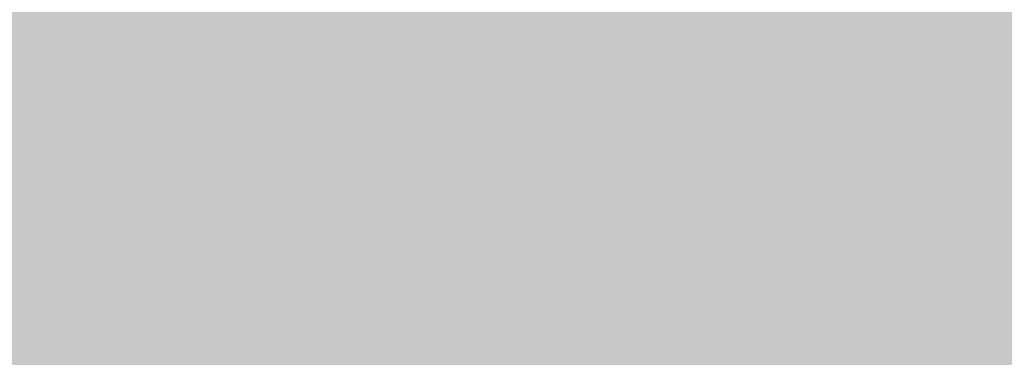
# Model space of a CAD drawing. Units: millimetres. Extents: x 0 to 2267, y 0 to 1823.
# Tile 74 of 256: x 1596.855 to 1600.369, y 1227.321 to 1228.528. Entities that reach past the tile are written whole.
import ezdxf

# ---------------------------------------------------------------- set-up
doc = ezdxf.new("R2010")
doc.units = ezdxf.units.MM
doc.header["$MEASUREMENT"] = 0
doc.layers.add('M-HATC', color=252, linetype='Continuous', lineweight=18)

msp = doc.modelspace()

# ---------------------------------------------------------------- hatches: boundary and pattern name
at = {"layer": 'M-HATC'}
h = msp.add_hatch(color=256, dxfattribs=at)
h.dxf.hatch_style = 1
h.paths.add_polyline_path([(2055.771, 1603.062), (1381.0868, 1603.062), (1381.0868, 1598.062), (2055.771, 1598.062)])
h.paths.add_polyline_path([(2055.771, 1598.062), (1381.0868, 1598.062), (1381.0868, 1593.062), (2055.771, 1593.062)])
h.paths.add_polyline_path([(2051.3074, 1536.7609), (1385.5504, 1536.7609), (1385.5504, 1526.7609), (1387.5504, 1526.7609), (1388.5366, 1525.0528), (1385.3319, 1521.2335), (1385.3319, 1521.2226), (2050.2542, 1522.7491), (2048.3212, 1525.0528), (2049.3074, 1526.7609), (2051.3074, 1526.7609)])
edge = h.paths.add_edge_path()
edge.add_arc((1847.5345, 1379.1492), 135, 222.603061, 222.890851, ccw=False)
edge.add_line((1748.1663, 1287.7656), (1683.0921, 1287.7656))
edge.add_arc((1583.7239, 1379.1492), 135, 317.109149, 317.396939, ccw=False)
edge.add_arc((1678.9686, 1290.6707), 5, 222.8909, 317.1091, ccw=False)
edge.add_arc((1774.2133, 1379.1492), 135, 222.603061, 222.890851, ccw=False)
edge.add_line((1674.8451, 1287.7656), (1609.7709, 1287.7656))
edge.add_arc((1510.4027, 1379.1492), 135, 317.109149, 317.396939, ccw=False)
edge.add_arc((1605.6474, 1290.6707), 5, 222.8909, 317.1091, ccw=False)
edge.add_arc((1700.8921, 1379.1492), 135, 222.603061, 222.890851, ccw=False)
edge.add_line((1601.5239, 1287.7656), (1536.4497, 1287.7656))
edge.add_arc((1437.0815, 1379.1492), 135, 317.109149, 317.396939, ccw=False)
edge.add_arc((1532.3262, 1290.6707), 5, 222.8909, 317.1091, ccw=False)
edge.add_arc((1627.5709, 1379.1492), 135, 222.603061, 222.890851, ccw=False)
edge.add_line((1528.2027, 1287.7656), (1505.9289, 1287.7656))
edge.add_spline(control_points=[(1505.9289, 1287.7656), (1504.2622, 1287.7656), (1504.2622, 1282.7656), (1505.9289, 1282.7656)], knot_values=[0, 0, 0, 0, 5, 5, 5, 5], degree=3, periodic=0)
edge.add_line((1505.9289, 1282.7656), (1930.9289, 1282.7656))
edge.add_spline(control_points=[(1930.9289, 1282.7656), (1932.5956, 1282.7656), (1932.5956, 1287.7656), (1930.9289, 1287.7656)], knot_values=[0, 0, 0, 0, 5, 5, 5, 5], degree=3, periodic=0)
edge.add_line((1930.9289, 1287.7656), (1903.0557, 1287.7656))
edge.add_arc((1803.6875, 1379.1492), 135, 317.109149, 317.396939, ccw=False)
edge.add_arc((1898.9322, 1290.6707), 5, 222.8909, 317.1091, ccw=False)
edge.add_arc((1994.1769, 1379.1492), 135, 222.603061, 222.890851, ccw=False)
edge.add_line((1894.8087, 1287.7656), (1829.7345, 1287.7656))
edge.add_arc((1730.3663, 1379.1492), 135, 317.109149, 317.396939, ccw=False)
edge.add_arc((1825.611, 1290.6707), 5, 222.8909, 317.1091, ccw=False)
edge.add_arc((1920.8557, 1379.1492), 135, 222.603061, 222.890851, ccw=False)
edge.add_line((1821.4875, 1287.7656), (1756.4133, 1287.7656))
edge.add_arc((1657.0451, 1379.1492), 135, 317.109149, 317.396939, ccw=False)
edge.add_arc((1752.2898, 1290.6707), 5, 222.8909, 317.1091, ccw=False)
edge = h.paths.add_edge_path()
edge.add_spline(control_points=[(1843.4289, 1227.2475), (1845.0956, 1227.2475), (1845.0956, 1232.2475), (1843.4289, 1232.2475)], knot_values=[0, 0, 0, 0, 5, 5, 5, 5], degree=3, periodic=0)
edge.add_line((1843.4289, 1232.2475), (1593.4289, 1232.2475))
edge.add_spline(control_points=[(1593.4289, 1232.2475), (1591.7622, 1232.2475), (1591.7622, 1227.2475), (1593.4289, 1227.2475)], knot_values=[0, 0, 0, 0, 5, 5, 5, 5], degree=3, periodic=0)
edge.add_line((1593.4289, 1227.2475), (1843.4289, 1227.2475))
h.paths.add_polyline_path([(1905.9289, 1127.4171), (1530.9289, 1127.4171, 0.414214), (1520.9289, 1117.4171), (1530.9289, 1117.4171), (1915.9289, 1117.4171, 0.414214)])
edge = h.paths.add_edge_path()
edge.add_arc((1397.0858, 1498.4078), 12.7299, 90.78215, 190.87871, ccw=False)
edge.add_line((1396.912, 1511.1365), (1428.0097, 1511.3488))
edge.add_line((1428.0097, 1511.3488), (1433.0097, 1511.3488))
edge.add_line((1433.0097, 1511.3488), (1434.439, 1511.3488))
edge.add_arc((1419.474, 1498.0804), 20, 41.561, 74.08211)
edge.add_line((1424.9592, 1517.3135), (1399.9351, 1517.2561))
edge.add_spline(control_points=[(1399.9307, 1517.2561), (1399.884, 1517.2131), (1399.8328, 1517.1689), (1399.7774, 1517.1236)], knot_values=[11.567499, 11.567499, 11.567499, 11.567499, 11.814249, 11.814249, 11.814249, 11.814249], degree=3, periodic=0)
edge.add_spline(control_points=[(1399.6328, 1517.0099), (1399.5831, 1516.9721), (1399.5307, 1516.9338), (1399.4759, 1516.8947)], knot_values=[11.167718, 11.167718, 11.167718, 11.167718, 11.365188, 11.365188, 11.365188, 11.365188], degree=3, periodic=0)
edge.add_spline(control_points=[(1399.3398, 1516.8001), (1399.1514, 1516.6719), (1398.9384, 1516.5377), (1398.704, 1516.3994)], knot_values=[10.376405, 10.376405, 10.376405, 10.376405, 11.00994, 11.00994, 11.00994, 11.00994], degree=3, periodic=0)
edge.add_spline(control_points=[(1398.6572, 1516.3719), (1398.5789, 1516.326), (1398.4983, 1516.2797), (1398.4155, 1516.2331)], knot_values=[10.125175, 10.125175, 10.125175, 10.125175, 10.334406, 10.334406, 10.334406, 10.334406], degree=3, periodic=0)
edge.add_spline(control_points=[(1398.2642, 1516.1487), (1398.196, 1516.1111), (1398.1263, 1516.0732), (1398.0555, 1516.0351)], knot_values=[9.832246, 9.832246, 9.832246, 9.832246, 9.999658, 9.999658, 9.999658, 9.999658], degree=3, periodic=0)
edge.add_spline(control_points=[(1397.9987, 1516.0048), (1397.7312, 1515.8621), (1397.446, 1515.7171), (1397.1466, 1515.5714)], knot_values=[9.161808, 9.161808, 9.161808, 9.161808, 9.787769, 9.787769, 9.787769, 9.787769], degree=3, periodic=0)
edge.add_spline(control_points=[(1397.1466, 1515.5714), (1396.8418, 1515.423), (1396.5222, 1515.274), (1396.1914, 1515.1262)], knot_values=[8.524455, 8.524455, 8.524455, 8.524455, 9.161808, 9.161808, 9.161808, 9.161808], degree=3, periodic=0)
edge.add_spline(control_points=[(1396.0777, 1515.0756), (1395.9854, 1515.0348), (1395.8922, 1514.994), (1395.7983, 1514.9534)], knot_values=[8.275193, 8.275193, 8.275193, 8.275193, 8.451726, 8.451726, 8.451726, 8.451726], degree=3, periodic=0)
edge.add_spline(control_points=[(1395.6018, 1514.8691), (1395.4997, 1514.8257), (1395.3968, 1514.7824), (1395.2932, 1514.7394)], knot_values=[7.962917, 7.962917, 7.962917, 7.962917, 8.152764, 8.152764, 8.152764, 8.152764], degree=3, periodic=0)
edge.add_spline(control_points=[(1395.2116, 1514.7057), (1394.8278, 1514.5475), (1394.4345, 1514.3929), (1394.0364, 1514.2442)], knot_values=[7.21254, 7.21254, 7.21254, 7.21254, 7.913148, 7.913148, 7.913148, 7.913148], degree=3, periodic=0)
edge.add_spline(control_points=[(1394.0364, 1514.2442), (1393.7076, 1514.1214), (1393.3754, 1514.0027), (1393.0427, 1513.8895)], knot_values=[6.633733, 6.633733, 6.633733, 6.633733, 7.21254, 7.21254, 7.21254, 7.21254], degree=3, periodic=0)
edge.add_spline(control_points=[(1392.8214, 1513.815), (1392.7198, 1513.7812), (1392.6181, 1513.7479), (1392.5166, 1513.7152)], knot_values=[6.328796, 6.328796, 6.328796, 6.328796, 6.505493, 6.505493, 6.505493, 6.505493], degree=3, periodic=0)
edge.add_spline(control_points=[(1392.5166, 1513.7152), (1392.3187, 1513.6515), (1392.1212, 1513.59), (1391.9244, 1513.531)], knot_values=[5.984605, 5.984605, 5.984605, 5.984605, 6.328796, 6.328796, 6.328796, 6.328796], degree=3, periodic=0)
edge.add_spline(control_points=[(1391.7915, 1513.4915), (1391.3122, 1513.3501), (1390.8384, 1513.2239), (1390.3784, 1513.1171)], knot_values=[5.066697, 5.066697, 5.066697, 5.066697, 5.907055, 5.907055, 5.907055, 5.907055], degree=3, periodic=0)
edge.add_spline(control_points=[(1390.3784, 1513.1171), (1390.1797, 1513.071), (1389.9836, 1513.0284), (1389.7907, 1512.9899)], knot_values=[4.70367, 4.70367, 4.70367, 4.70367, 5.066695, 5.066695, 5.066695, 5.066695], degree=3, periodic=0)
edge.add_spline(control_points=[(1389.422, 1512.9204), (1389.2459, 1512.8892), (1389.0729, 1512.8617), (1388.9036, 1512.8381)], knot_values=[4.130571, 4.130571, 4.130571, 4.130571, 4.469816, 4.469816, 4.469816, 4.469816], degree=3, periodic=0)
edge.add_spline(control_points=[(1388.9036, 1512.8381), (1388.591, 1512.7946), (1388.2911, 1512.7644), (1388.0071, 1512.7494)], knot_values=[3.504031, 3.504031, 3.504031, 3.504031, 4.130571, 4.130571, 4.130571, 4.130571], degree=3, periodic=0)
edge.add_spline(control_points=[(1387.9356, 1512.7459), (1387.8538, 1512.7423), (1387.7733, 1512.74), (1387.6944, 1512.739)], knot_values=[3.268866, 3.268866, 3.268866, 3.268866, 3.451164, 3.451164, 3.451164, 3.451164], degree=3, periodic=0)
edge.add_spline(control_points=[(1387.3351, 1512.7443), (1387.2076, 1512.7499), (1387.0847, 1512.7597), (1386.967, 1512.7739)], knot_values=[2.670686, 2.670686, 2.670686, 2.670686, 2.984, 2.984, 2.984, 2.984], degree=3, periodic=0)
edge.add_spline(control_points=[(1386.8327, 1512.7922), (1386.8209, 1512.7941), (1386.8092, 1512.7959), (1386.7975, 1512.7979)], knot_values=[2.516981, 2.516981, 2.516981, 2.516981, 2.549528, 2.549528, 2.549528, 2.549528], degree=3, periodic=0)
edge.add_spline(control_points=[(1386.4526, 1512.8735), (1386.4257, 1512.881), (1386.3993, 1512.889), (1386.3733, 1512.8972)], knot_values=[2.095869, 2.095869, 2.095869, 2.095869, 2.17941, 2.17941, 2.17941, 2.17941], degree=3, periodic=0)
edge.add_spline(control_points=[(1386.0691, 1513.0189), (1386.0634, 1513.0217), (1386.0577, 1513.0246), (1386.052, 1513.0275)], knot_values=[1.72453, 1.72453, 1.72453, 1.72453, 1.745933, 1.745933, 1.745933, 1.745933], degree=3, periodic=0)
edge.add_arc((1399.474, 1498.0804), 20, 131.82432, 180)
edge.add_arc((1630.3336, 1505.5484), 250.9708, 181.705176, 236.427975)
edge.add_arc((1605.3399, 1483.3044), 218.7822, 238.660829, 243.34961)
edge.add_arc((1647.0911, 1510.3592), 262.8986, 183.129836, 237.853442, ccw=False)
h.paths.add_polyline_path([(1406.5369, 1391.9644, 0.149382), (1491.5506, 1296.4418, -0.129517)], flags=17)
edge = h.paths.add_edge_path()
edge.add_arc((2037.3838, 1498.0804), 20, 0, 48.26587)
edge.add_spline(control_points=[(2050.6973, 1513.0052), (2050.6512, 1512.9847), (2050.6034, 1512.9655), (2050.5539, 1512.9477)], knot_values=[1.835652, 1.835652, 1.835652, 1.835652, 2.000781, 2.000781, 2.000781, 2.000781], degree=3, periodic=0)
edge.add_spline(control_points=[(2050.4616, 1512.9166), (2050.479, 1512.9221), (2050.4963, 1512.9277), (2050.5133, 1512.9335)], knot_values=[2.045477, 2.045477, 2.045477, 2.045477, 2.101389, 2.101389, 2.101389, 2.101389], degree=3, periodic=0)
edge.add_spline(control_points=[(2050.129, 1512.8342), (2050.1984, 1512.8473), (2050.2657, 1512.8623), (2050.3308, 1512.8792)], knot_values=[2.237629, 2.237629, 2.237629, 2.237629, 2.435841, 2.435841, 2.435841, 2.435841], degree=3, periodic=0)
edge.add_spline(control_points=[(2050.0946, 1512.8278), (2050.1061, 1512.8299), (2050.1176, 1512.832), (2050.129, 1512.8342)], knot_values=[2.435841, 2.435841, 2.435841, 2.435841, 2.468321, 2.468321, 2.468321, 2.468321], degree=3, periodic=0)
edge.add_spline(control_points=[(2049.7843, 1512.7851), (2049.8552, 1512.7922), (2049.9243, 1512.8008), (2049.9917, 1512.8109)], knot_values=[2.563852, 2.563852, 2.563852, 2.563852, 2.748541, 2.748541, 2.748541, 2.748541], degree=3, periodic=0)
edge.add_spline(control_points=[(2049.4052, 1512.7617), (2049.5364, 1512.7653), (2049.6629, 1512.773), (2049.7843, 1512.7851)], knot_values=[2.748541, 2.748541, 2.748541, 2.748541, 3.064882, 3.064882, 3.064882, 3.064882], degree=3, periodic=0)
edge.add_spline(control_points=[(2049.1698, 1512.7597), (2049.2336, 1512.7591), (2049.2965, 1512.7594), (2049.3584, 1512.7606)], knot_values=[3.102309, 3.102309, 3.102309, 3.102309, 3.2503, 3.2503, 3.2503, 3.2503], degree=3, periodic=0)
edge.add_spline(control_points=[(2048.8573, 1512.7691), (2048.9638, 1512.7638), (2049.068, 1512.7606), (2049.1698, 1512.7597)], knot_values=[3.2503, 3.2503, 3.2503, 3.2503, 3.486069, 3.486069, 3.486069, 3.486069], degree=3, periodic=0)
edge.add_spline(control_points=[(2048.6924, 1512.7789), (2048.3729, 1512.8009), (2048.0345, 1512.8411), (2047.6817, 1512.897)], knot_values=[3.606429, 3.606429, 3.606429, 3.606429, 4.2989, 4.2989, 4.2989, 4.2989], degree=3, periodic=0)
edge.add_spline(control_points=[(2047.6817, 1512.897), (2047.5458, 1512.9185), (2047.4077, 1512.9424), (2047.2678, 1512.9685)], knot_values=[4.2989, 4.2989, 4.2989, 4.2989, 4.565769, 4.565769, 4.565769, 4.565769], degree=3, periodic=0)
edge.add_spline(control_points=[(2047.2678, 1512.9685), (2047.1449, 1512.9914), (2047.0207, 1513.016), (2046.8951, 1513.0422)], knot_values=[4.565769, 4.565769, 4.565769, 4.565769, 4.799971, 4.799971, 4.799971, 4.799971], degree=3, periodic=0)
edge.add_spline(control_points=[(2046.8951, 1513.0422), (2046.5286, 1513.1188), (2046.1513, 1513.209), (2045.7676, 1513.3107)], knot_values=[4.799971, 4.799971, 4.799971, 4.799971, 5.483718, 5.483718, 5.483718, 5.483718], degree=3, periodic=0)
edge.add_spline(control_points=[(2045.7676, 1513.3107), (2045.3724, 1513.4154), (2044.9704, 1513.5322), (2044.5662, 1513.6588)], knot_values=[5.483718, 5.483718, 5.483718, 5.483718, 6.187866, 6.187866, 6.187866, 6.187866], degree=3, periodic=0)
edge.add_spline(control_points=[(2044.5662, 1513.6588), (2044.4149, 1513.7061), (2044.2633, 1513.7549), (2044.1116, 1513.8048)], knot_values=[6.187866, 6.187866, 6.187866, 6.187866, 6.451551, 6.451551, 6.451551, 6.451551], degree=3, periodic=0)
edge.add_spline(control_points=[(2044.1116, 1513.8048), (2043.9967, 1513.8427), (2043.8817, 1513.8813), (2043.7668, 1513.9205)], knot_values=[6.451551, 6.451551, 6.451551, 6.451551, 6.651434, 6.651434, 6.651434, 6.651434], degree=3, periodic=0)
edge.add_spline(control_points=[(2043.7668, 1513.9205), (2043.3716, 1514.0554), (2042.9774, 1514.1979), (2042.5886, 1514.3458)], knot_values=[6.651434, 6.651434, 6.651434, 6.651434, 7.338879, 7.338879, 7.338879, 7.338879], degree=3, periodic=0)
edge.add_spline(control_points=[(2042.5886, 1514.3458), (2042.1643, 1514.5071), (2041.7465, 1514.6749), (2041.3409, 1514.846)], knot_values=[7.338879, 7.338879, 7.338879, 7.338879, 8.089209, 8.089209, 8.089209, 8.089209], degree=3, periodic=0)
edge.add_spline(control_points=[(2041.3409, 1514.846), (2041.1028, 1514.9465), (2040.869, 1515.0481), (2040.6405, 1515.1502)], knot_values=[8.089209, 8.089209, 8.089209, 8.089209, 8.529587, 8.529587, 8.529587, 8.529587], degree=3, periodic=0)
edge.add_spline(control_points=[(2040.51, 1515.2089), (2040.0824, 1515.4022), (2039.6747, 1515.5971), (2039.295, 1515.7894)], knot_values=[8.613818, 8.613818, 8.613818, 8.613818, 9.44571, 9.44571, 9.44571, 9.44571], degree=3, periodic=0)
edge.add_spline(control_points=[(2039.295, 1515.7894), (2039.0618, 1515.9075), (2038.8391, 1516.0246), (2038.6288, 1516.1398)], knot_values=[9.44571, 9.44571, 9.44571, 9.44571, 9.956404, 9.956404, 9.956404, 9.956404], degree=3, periodic=0)
edge.add_spline(control_points=[(2038.6288, 1516.1398), (2038.5187, 1516.2001), (2038.4121, 1516.2598), (2038.309, 1516.3189)], knot_values=[9.956404, 9.956404, 9.956404, 9.956404, 10.223542, 10.223542, 10.223542, 10.223542], degree=3, periodic=0)
edge.add_spline(control_points=[(2038.309, 1516.3189), (2038.2138, 1516.3735), (2038.1216, 1516.4276), (2038.0328, 1516.481)], knot_values=[10.223542, 10.223542, 10.223542, 10.223542, 10.47051, 10.47051, 10.47051, 10.47051], degree=3, periodic=0)
edge.add_spline(control_points=[(2038.0328, 1516.481), (2037.7855, 1516.6296), (2037.5639, 1516.773), (2037.3722, 1516.909)], knot_values=[10.47051, 10.47051, 10.47051, 10.47051, 11.15767, 11.15767, 11.15767, 11.15767], degree=3, periodic=0)
edge.add_spline(control_points=[(2037.3722, 1516.909), (2037.2789, 1516.9752), (2037.1927, 1517.0396), (2037.1142, 1517.102)], knot_values=[11.15767, 11.15767, 11.15767, 11.15767, 11.49227, 11.49227, 11.49227, 11.49227], degree=3, periodic=0)
edge.add_spline(control_points=[(2036.8564, 1517.3259), (2036.9148, 1517.2692), (2036.9814, 1517.2103), (2037.0557, 1517.1492)], knot_values=[11.577341, 11.577341, 11.577341, 11.577341, 11.91035, 11.91035, 11.91035, 11.91035], degree=3, periodic=0)
edge.add_spline(control_points=[(2036.8074, 1517.3748), (2036.823, 1517.3587), (2036.8393, 1517.3424), (2036.8564, 1517.3259)], knot_values=[11.91035, 11.91035, 11.91035, 11.91035, 12.007402, 12.007402, 12.007402, 12.007402], degree=3, periodic=0)
edge.add_spline(control_points=[(2036.7017, 1517.494), (2036.7104, 1517.483), (2036.7196, 1517.4719), (2036.7291, 1517.4606)], knot_values=[12.184155, 12.184155, 12.184155, 12.184155, 12.255409, 12.255409, 12.255409, 12.255409], degree=3, periodic=0)
edge.add_spline(control_points=[(2036.6159, 1517.6205), (2036.62, 1517.613), (2036.6243, 1517.6055), (2036.6289, 1517.5979)], knot_values=[12.487913, 12.487913, 12.487913, 12.487913, 12.541035, 12.541035, 12.541035, 12.541035], degree=3, periodic=0)
edge.add_spline(control_points=[(2036.5635, 1517.786), (2036.5637, 1517.7794), (2036.5642, 1517.7726), (2036.565, 1517.7658)], knot_values=[12.911761, 12.911761, 12.911761, 12.911761, 12.968286, 12.968286, 12.968286, 12.968286], degree=3, periodic=0)
edge.add_spline(control_points=[(2036.6166, 1517.9304), (2036.6125, 1517.9259), (2036.6086, 1517.9212), (2036.6049, 1517.9165)], knot_values=[13.382527, 13.382527, 13.382527, 13.382527, 13.433791, 13.433791, 13.433791, 13.433791], degree=3, periodic=0)
edge.add_spline(control_points=[(2036.749, 1518.017), (2036.7361, 1518.0116), (2036.7239, 1518.006), (2036.7124, 1518.0002)], knot_values=[13.726299, 13.726299, 13.726299, 13.726299, 13.809928, 13.809928, 13.809928, 13.809928], degree=3, periodic=0)
edge.add_spline(control_points=[(2036.8604, 1518.0528), (2036.8386, 1518.0474), (2036.8181, 1518.0416), (2036.7988, 1518.0353)], knot_values=[13.910887, 13.910887, 13.910887, 13.910887, 14.02153, 14.02153, 14.02153, 14.02153], degree=3, periodic=0)
edge.add_line((2036.9639, 1518.0804), (2032.3838, 1518.0804))
edge.add_line((2032.3838, 1518.0804), (2027.3838, 1518.0804))
edge.add_line((2027.3838, 1518.0804), (2022.3838, 1518.0804))
edge.add_line((2022.3838, 1518.0804), (2017.3838, 1518.0804))
edge.add_arc((2017.3838, 1498.0804), 20, 90, 138.439)
edge.add_line((2002.4188, 1511.3488), (2003.8481, 1511.3488))
edge.add_line((2003.8481, 1511.3488), (2008.8481, 1511.3488))
edge.add_line((2008.8481, 1511.3488), (2039.772, 1511.1377))
edge.add_arc((2039.772, 1498.4078), 12.7299, -10.87871, 90, ccw=False)
edge.add_arc((1789.7668, 1510.3592), 262.8986, 302.146558, 356.870164, ccw=False)
edge.add_arc((1831.5179, 1483.3044), 218.7822, 296.65039, 301.339171)
edge.add_arc((1806.5242, 1505.5484), 250.9708, 303.572025, 358.294824)
h.paths.add_polyline_path([(2030.321, 1391.9644, -0.129517), (1945.3072, 1296.4418, 0.149382)], flags=17)
edge = h.paths.add_edge_path()
edge.add_spline(control_points=[(2037.2464, 1518.0821), (2037.2898, 1518.081), (2037.3355, 1518.0804), (2037.3838, 1518.0804)], knot_values=[0.000012, 0.000012, 0.000012, 0.000012, 0.144754, 0.144754, 0.144754, 0.144754], degree=3, periodic=0)
edge.add_line((2037.3357, 1518.0804), (2037.0096, 1518.0804))
edge.add_spline(control_points=[(2037.0096, 1518.0804), (2036.9822, 1518.0768), (2036.956, 1518.0727), (2036.9312, 1518.0681)], knot_values=[14.13465, 14.13465, 14.13465, 14.13465, 14.247197, 14.247197, 14.247197, 14.247197], degree=3, periodic=0)
edge.add_spline(control_points=[(2036.9312, 1518.0681), (2036.9276, 1518.0674), (2036.9241, 1518.0667), (2036.9205, 1518.0661)], knot_values=[14.118315, 14.118315, 14.118315, 14.118315, 14.13465, 14.13465, 14.13465, 14.13465], degree=3, periodic=0)
edge.add_spline(control_points=[(2036.9205, 1518.0661), (2036.9118, 1518.0644), (2036.9032, 1518.0626), (2036.8948, 1518.0608)], knot_values=[14.078086, 14.078086, 14.078086, 14.078086, 14.118315, 14.118315, 14.118315, 14.118315], degree=3, periodic=0)
edge.add_spline(control_points=[(2036.8948, 1518.0608), (2036.883, 1518.0583), (2036.8716, 1518.0556), (2036.8604, 1518.0528)], knot_values=[14.02153, 14.02153, 14.02153, 14.02153, 14.078086, 14.078086, 14.078086, 14.078086], degree=3, periodic=0)
edge.add_spline(control_points=[(2036.8604, 1518.0528), (2036.8386, 1518.0474), (2036.8181, 1518.0416), (2036.7988, 1518.0353)], knot_values=[13.910887, 13.910887, 13.910887, 13.910887, 14.02153, 14.02153, 14.02153, 14.02153], degree=3, periodic=0)
edge.add_spline(control_points=[(2036.7988, 1518.0353), (2036.7981, 1518.035), (2036.7974, 1518.0348), (2036.7967, 1518.0346)], knot_values=[13.906906, 13.906906, 13.906906, 13.906906, 13.910887, 13.910887, 13.910887, 13.910887], degree=3, periodic=0)
edge.add_spline(control_points=[(2036.7967, 1518.0346), (2036.7882, 1518.0318), (2036.7799, 1518.0289), (2036.7719, 1518.0259)], knot_values=[13.857826, 13.857826, 13.857826, 13.857826, 13.906906, 13.906906, 13.906906, 13.906906], degree=3, periodic=0)
edge.add_spline(control_points=[(2036.7719, 1518.0259), (2036.764, 1518.023), (2036.7564, 1518.02), (2036.749, 1518.017)], knot_values=[13.809928, 13.809928, 13.809928, 13.809928, 13.857826, 13.857826, 13.857826, 13.857826], degree=3, periodic=0)
edge.add_spline(control_points=[(2036.749, 1518.017), (2036.7361, 1518.0116), (2036.7239, 1518.006), (2036.7124, 1518.0002)], knot_values=[13.726299, 13.726299, 13.726299, 13.726299, 13.809928, 13.809928, 13.809928, 13.809928], degree=3, periodic=0)
edge.add_spline(control_points=[(2036.7124, 1518.0002), (2036.7121, 1518), (2036.7118, 1517.9999), (2036.7115, 1517.9997)], knot_values=[13.723993, 13.723993, 13.723993, 13.723993, 13.726299, 13.726299, 13.726299, 13.726299], degree=3, periodic=0)
edge.add_spline(control_points=[(2036.7115, 1517.9997), (2036.7063, 1517.9971), (2036.7013, 1517.9944), (2036.6965, 1517.9917)], knot_values=[13.686536, 13.686536, 13.686536, 13.686536, 13.723993, 13.723993, 13.723993, 13.723993], degree=3, periodic=0)
edge.add_spline(control_points=[(2036.6965, 1517.9917), (2036.6919, 1517.9891), (2036.6874, 1517.9865), (2036.6831, 1517.9839)], knot_values=[13.651251, 13.651251, 13.651251, 13.651251, 13.686536, 13.686536, 13.686536, 13.686536], degree=3, periodic=0)
edge.add_spline(control_points=[(2036.6831, 1517.9839), (2036.6764, 1517.9798), (2036.67, 1517.9757), (2036.6639, 1517.9714)], knot_values=[13.596804, 13.596804, 13.596804, 13.596804, 13.651251, 13.651251, 13.651251, 13.651251], degree=3, periodic=0)
edge.add_spline(control_points=[(2036.6639, 1517.9714), (2036.6636, 1517.9712), (2036.6633, 1517.9709), (2036.6629, 1517.9707)], knot_values=[13.593956, 13.593956, 13.593956, 13.593956, 13.596804, 13.596804, 13.596804, 13.596804], degree=3, periodic=0)
edge.add_spline(control_points=[(2036.6629, 1517.9707), (2036.6603, 1517.9689), (2036.6577, 1517.967), (2036.6552, 1517.9651)], knot_values=[13.570322, 13.570322, 13.570322, 13.570322, 13.593956, 13.593956, 13.593956, 13.593956], degree=3, periodic=0)
edge.add_spline(control_points=[(2036.6552, 1517.9651), (2036.6525, 1517.9631), (2036.6499, 1517.9611), (2036.6474, 1517.9591)], knot_values=[13.545477, 13.545477, 13.545477, 13.545477, 13.570322, 13.570322, 13.570322, 13.570322], degree=3, periodic=0)
edge.add_spline(control_points=[(2036.6474, 1517.9591), (2036.6472, 1517.9589), (2036.6471, 1517.9588), (2036.6469, 1517.9587)], knot_values=[13.543931, 13.543931, 13.543931, 13.543931, 13.545477, 13.545477, 13.545477, 13.545477], degree=3, periodic=0)
edge.add_spline(control_points=[(2036.6469, 1517.9587), (2036.6412, 1517.9541), (2036.6358, 1517.9494), (2036.6307, 1517.9447)], knot_values=[13.488237, 13.488237, 13.488237, 13.488237, 13.543931, 13.543931, 13.543931, 13.543931], degree=3, periodic=0)
edge.add_spline(control_points=[(2036.6307, 1517.9447), (2036.6282, 1517.9423), (2036.6257, 1517.9399), (2036.6233, 1517.9374)], knot_values=[13.460307, 13.460307, 13.460307, 13.460307, 13.488237, 13.488237, 13.488237, 13.488237], degree=3, periodic=0)
edge.add_spline(control_points=[(2036.6233, 1517.9374), (2036.6215, 1517.9356), (2036.6198, 1517.9338), (2036.6181, 1517.932)], knot_values=[13.439712, 13.439712, 13.439712, 13.439712, 13.460307, 13.460307, 13.460307, 13.460307], degree=3, periodic=0)
edge.add_spline(control_points=[(2036.6181, 1517.932), (2036.6176, 1517.9315), (2036.6171, 1517.9309), (2036.6166, 1517.9304)], knot_values=[13.433791, 13.433791, 13.433791, 13.433791, 13.439712, 13.439712, 13.439712, 13.439712], degree=3, periodic=0)
edge.add_spline(control_points=[(2036.6166, 1517.9304), (2036.6125, 1517.9259), (2036.6086, 1517.9212), (2036.6049, 1517.9165)], knot_values=[13.382527, 13.382527, 13.382527, 13.382527, 13.433791, 13.433791, 13.433791, 13.433791], degree=3, periodic=0)
edge.add_spline(control_points=[(2036.6049, 1517.9165), (2036.6026, 1517.9135), (2036.6004, 1517.9104), (2036.5982, 1517.9074)], knot_values=[13.350017, 13.350017, 13.350017, 13.350017, 13.382527, 13.382527, 13.382527, 13.382527], degree=3, periodic=0)
edge.add_spline(control_points=[(2036.5982, 1517.9074), (2036.5972, 1517.9059), (2036.5962, 1517.9043), (2036.5952, 1517.9028)], knot_values=[13.333922, 13.333922, 13.333922, 13.333922, 13.350017, 13.350017, 13.350017, 13.350017], degree=3, periodic=0)
edge.add_spline(control_points=[(2036.5952, 1517.9028), (2036.5945, 1517.9018), (2036.5939, 1517.9009), (2036.5933, 1517.8999)], knot_values=[13.323828, 13.323828, 13.323828, 13.323828, 13.333922, 13.333922, 13.333922, 13.333922], degree=3, periodic=0)
edge.add_spline(control_points=[(2036.5933, 1517.8999), (2036.5905, 1517.8955), (2036.5879, 1517.8909), (2036.5855, 1517.8864)], knot_values=[13.277545, 13.277545, 13.277545, 13.277545, 13.323828, 13.323828, 13.323828, 13.323828], degree=3, periodic=0)
edge.add_spline(control_points=[(2036.5855, 1517.8864), (2036.5836, 1517.8827), (2036.5817, 1517.8789), (2036.5801, 1517.8751)], knot_values=[13.240119, 13.240119, 13.240119, 13.240119, 13.277545, 13.277545, 13.277545, 13.277545], degree=3, periodic=0)
edge.add_spline(control_points=[(2036.5801, 1517.8751), (2036.5795, 1517.8739), (2036.579, 1517.8727), (2036.5785, 1517.8715)], knot_values=[13.228211, 13.228211, 13.228211, 13.228211, 13.240119, 13.240119, 13.240119, 13.240119], degree=3, periodic=0)
edge.add_spline(control_points=[(2036.5785, 1517.8715), (2036.578, 1517.8702), (2036.5774, 1517.869), (2036.5769, 1517.8677)], knot_values=[13.215717, 13.215717, 13.215717, 13.215717, 13.228211, 13.228211, 13.228211, 13.228211], degree=3, periodic=0)
edge.add_spline(control_points=[(2036.5769, 1517.8677), (2036.5755, 1517.864), (2036.5741, 1517.8603), (2036.5729, 1517.8565)], knot_values=[13.179847, 13.179847, 13.179847, 13.179847, 13.215717, 13.215717, 13.215717, 13.215717], degree=3, periodic=0)
edge.add_spline(control_points=[(2036.5729, 1517.8565), (2036.5713, 1517.8515), (2036.5699, 1517.8464), (2036.5687, 1517.8413)], knot_values=[13.132017, 13.132017, 13.132017, 13.132017, 13.179847, 13.179847, 13.179847, 13.179847], degree=3, periodic=0)
edge.add_spline(control_points=[(2036.5687, 1517.8413), (2036.5684, 1517.8402), (2036.5682, 1517.8392), (2036.568, 1517.8382)], knot_values=[13.122482, 13.122482, 13.122482, 13.122482, 13.132017, 13.132017, 13.132017, 13.132017], degree=3, periodic=0)
edge.add_spline(control_points=[(2036.568, 1517.8382), (2036.5676, 1517.8363), (2036.5672, 1517.8345), (2036.5669, 1517.8327)], knot_values=[13.105592, 13.105592, 13.105592, 13.105592, 13.122482, 13.122482, 13.122482, 13.122482], degree=3, periodic=0)
edge.add_spline(control_points=[(2036.5669, 1517.8327), (2036.5662, 1517.8292), (2036.5657, 1517.8257), (2036.5652, 1517.8222)], knot_values=[13.074063, 13.074063, 13.074063, 13.074063, 13.105592, 13.105592, 13.105592, 13.105592], degree=3, periodic=0)
edge.add_spline(control_points=[(2036.5652, 1517.8222), (2036.5652, 1517.8222), (2036.5652, 1517.8222), (2036.5652, 1517.8222)], knot_values=[13.074043, 13.074043, 13.074043, 13.074043, 13.074063, 13.074063, 13.074063, 13.074063], degree=3, periodic=0)
edge.add_spline(control_points=[(2036.5652, 1517.8222), (2036.5644, 1517.8164), (2036.5639, 1517.8106), (2036.5636, 1517.8046)], knot_values=[13.021884, 13.021884, 13.021884, 13.021884, 13.074043, 13.074043, 13.074043, 13.074043], degree=3, periodic=0)
edge.add_spline(control_points=[(2036.5636, 1517.8046), (2036.5636, 1517.804), (2036.5636, 1517.8034), (2036.5635, 1517.8028)], knot_values=[13.01674, 13.01674, 13.01674, 13.01674, 13.021884, 13.021884, 13.021884, 13.021884], degree=3, periodic=0)
edge.add_spline(control_points=[(2036.5635, 1517.8028), (2036.5634, 1517.8005), (2036.5634, 1517.7982), (2036.5634, 1517.7958)], knot_values=[12.996438, 12.996438, 12.996438, 12.996438, 13.01674, 13.01674, 13.01674, 13.01674], degree=3, periodic=0)
edge.add_spline(control_points=[(2036.5634, 1517.7958), (2036.5633, 1517.7926), (2036.5634, 1517.7893), (2036.5635, 1517.786)], knot_values=[12.968286, 12.968286, 12.968286, 12.968286, 12.996438, 12.996438, 12.996438, 12.996438], degree=3, periodic=0)
edge.add_spline(control_points=[(2036.5635, 1517.786), (2036.5637, 1517.7794), (2036.5642, 1517.7726), (2036.565, 1517.7658)], knot_values=[12.911761, 12.911761, 12.911761, 12.911761, 12.968286, 12.968286, 12.968286, 12.968286], degree=3, periodic=0)
edge.add_spline(control_points=[(2036.565, 1517.7658), (2036.565, 1517.7657), (2036.565, 1517.7656), (2036.565, 1517.7656)], knot_values=[12.911017, 12.911017, 12.911017, 12.911017, 12.911761, 12.911761, 12.911761, 12.911761], degree=3, periodic=0)
edge.add_spline(control_points=[(2036.565, 1517.7656), (2036.5654, 1517.7625), (2036.5658, 1517.7593), (2036.5663, 1517.7562)], knot_values=[12.88528, 12.88528, 12.88528, 12.88528, 12.911017, 12.911017, 12.911017, 12.911017], degree=3, periodic=0)
edge.add_spline(control_points=[(2036.5663, 1517.7562), (2036.5667, 1517.7534), (2036.5672, 1517.7506), (2036.5677, 1517.7478)], knot_values=[12.862519, 12.862519, 12.862519, 12.862519, 12.88528, 12.88528, 12.88528, 12.88528], degree=3, periodic=0)
edge.add_spline(control_points=[(2036.5677, 1517.7478), (2036.5678, 1517.7474), (2036.5679, 1517.7469), (2036.568, 1517.7465)], knot_values=[12.858885, 12.858885, 12.858885, 12.858885, 12.862519, 12.862519, 12.862519, 12.862519], degree=3, periodic=0)
edge.add_spline(control_points=[(2036.568, 1517.7465), (2036.5692, 1517.7399), (2036.5707, 1517.7332), (2036.5724, 1517.7264)], knot_values=[12.8053, 12.8053, 12.8053, 12.8053, 12.858885, 12.858885, 12.858885, 12.858885], degree=3, periodic=0)
edge.add_spline(control_points=[(2036.5724, 1517.7264), (2036.5734, 1517.7226), (2036.5745, 1517.7187), (2036.5756, 1517.7149)], knot_values=[12.775176, 12.775176, 12.775176, 12.775176, 12.8053, 12.8053, 12.8053, 12.8053], degree=3, periodic=0)
edge.add_spline(control_points=[(2036.5756, 1517.7149), (2036.5763, 1517.7125), (2036.577, 1517.7102), (2036.5778, 1517.7078)], knot_values=[12.756759, 12.756759, 12.756759, 12.756759, 12.775176, 12.775176, 12.775176, 12.775176], degree=3, periodic=0)
edge.add_spline(control_points=[(2036.5778, 1517.7078), (2036.5781, 1517.7067), (2036.5784, 1517.7057), (2036.5787, 1517.7047)], knot_values=[12.748742, 12.748742, 12.748742, 12.748742, 12.756759, 12.756759, 12.756759, 12.756759], degree=3, periodic=0)
edge.add_spline(control_points=[(2036.5787, 1517.7047), (2036.5808, 1517.6983), (2036.5831, 1517.6919), (2036.5856, 1517.6854)], knot_values=[12.69959, 12.69959, 12.69959, 12.69959, 12.748742, 12.748742, 12.748742, 12.748742], degree=3, periodic=0)
edge.add_spline(control_points=[(2036.5856, 1517.6854), (2036.5876, 1517.68), (2036.5898, 1517.6746), (2036.5921, 1517.6692)], knot_values=[12.659038, 12.659038, 12.659038, 12.659038, 12.69959, 12.69959, 12.69959, 12.69959], degree=3, periodic=0)
edge.add_spline(control_points=[(2036.5921, 1517.6692), (2036.594, 1517.6648), (2036.5959, 1517.6605), (2036.5979, 1517.6561)], knot_values=[12.626806, 12.626806, 12.626806, 12.626806, 12.659038, 12.659038, 12.659038, 12.659038], degree=3, periodic=0)
edge.add_spline(control_points=[(2036.5979, 1517.6561), (2036.5984, 1517.6551), (2036.5989, 1517.6541), (2036.5993, 1517.6531)], knot_values=[12.619394, 12.619394, 12.619394, 12.619394, 12.626806, 12.626806, 12.626806, 12.626806], degree=3, periodic=0)
edge.add_spline(control_points=[(2036.5993, 1517.6531), (2036.6043, 1517.6424), (2036.6099, 1517.6315), (2036.6159, 1517.6205)], knot_values=[12.541039, 12.541039, 12.541039, 12.541039, 12.619394, 12.619394, 12.619394, 12.619394], degree=3, periodic=0)
edge.add_spline(control_points=[(2036.6159, 1517.6205), (2036.6159, 1517.6205), (2036.6159, 1517.6205), (2036.6159, 1517.6205)], knot_values=[12.541035, 12.541035, 12.541035, 12.541035, 12.541039, 12.541039, 12.541039, 12.541039], degree=3, periodic=0)
edge.add_spline(control_points=[(2036.6159, 1517.6205), (2036.62, 1517.613), (2036.6243, 1517.6055), (2036.6289, 1517.5979)], knot_values=[12.487913, 12.487913, 12.487913, 12.487913, 12.541035, 12.541035, 12.541035, 12.541035], degree=3, periodic=0)
edge.add_spline(control_points=[(2036.6289, 1517.5979), (2036.6326, 1517.5916), (2036.6365, 1517.5853), (2036.6406, 1517.5789)], knot_values=[12.443982, 12.443982, 12.443982, 12.443982, 12.487913, 12.487913, 12.487913, 12.487913], degree=3, periodic=0)
edge.add_spline(control_points=[(2036.6406, 1517.5789), (2036.6414, 1517.5776), (2036.6423, 1517.5763), (2036.6431, 1517.5749)], knot_values=[12.434996, 12.434996, 12.434996, 12.434996, 12.443982, 12.443982, 12.443982, 12.443982], degree=3, periodic=0)
edge.add_spline(control_points=[(2036.6431, 1517.5749), (2036.6531, 1517.5596), (2036.6639, 1517.5439), (2036.6756, 1517.528)], knot_values=[12.329647, 12.329647, 12.329647, 12.329647, 12.434996, 12.434996, 12.434996, 12.434996], degree=3, periodic=0)
edge.add_spline(control_points=[(2036.6756, 1517.528), (2036.6839, 1517.5168), (2036.6925, 1517.5055), (2036.7017, 1517.494)], knot_values=[12.255409, 12.255409, 12.255409, 12.255409, 12.329647, 12.329647, 12.329647, 12.329647], degree=3, periodic=0)
edge.add_spline(control_points=[(2036.7017, 1517.494), (2036.7104, 1517.483), (2036.7196, 1517.4719), (2036.7291, 1517.4606)], knot_values=[12.184155, 12.184155, 12.184155, 12.184155, 12.255409, 12.255409, 12.255409, 12.255409], degree=3, periodic=0)
edge.add_spline(control_points=[(2036.7291, 1517.4606), (2036.7436, 1517.4435), (2036.759, 1517.4262), (2036.7753, 1517.4085)], knot_values=[12.075961, 12.075961, 12.075961, 12.075961, 12.184155, 12.184155, 12.184155, 12.184155], degree=3, periodic=0)
edge.add_spline(control_points=[(2036.7753, 1517.4085), (2036.7763, 1517.4075), (2036.7773, 1517.4064), (2036.7783, 1517.4054)], knot_values=[12.069502, 12.069502, 12.069502, 12.069502, 12.075961, 12.075961, 12.075961, 12.075961], degree=3, periodic=0)
edge.add_spline(control_points=[(2036.7783, 1517.4054), (2036.7877, 1517.3953), (2036.7974, 1517.385), (2036.8074, 1517.3748)], knot_values=[12.007402, 12.007402, 12.007402, 12.007402, 12.069502, 12.069502, 12.069502, 12.069502], degree=3, periodic=0)
edge.add_spline(control_points=[(2036.8074, 1517.3748), (2036.823, 1517.3587), (2036.8393, 1517.3424), (2036.8564, 1517.3259)], knot_values=[11.91035, 11.91035, 11.91035, 11.91035, 12.007402, 12.007402, 12.007402, 12.007402], degree=3, periodic=0)
edge.add_spline(control_points=[(2036.8564, 1517.3259), (2036.9148, 1517.2692), (2036.9814, 1517.2103), (2037.0557, 1517.1492)], knot_values=[11.577341, 11.577341, 11.577341, 11.577341, 11.91035, 11.91035, 11.91035, 11.91035], degree=3, periodic=0)
edge.add_spline(control_points=[(2037.0557, 1517.1492), (2037.0747, 1517.1336), (2037.0942, 1517.1179), (2037.1142, 1517.102)], knot_values=[11.49227, 11.49227, 11.49227, 11.49227, 11.577341, 11.577341, 11.577341, 11.577341], degree=3, periodic=0)
edge.add_spline(control_points=[(2037.1142, 1517.102), (2037.1927, 1517.0396), (2037.2789, 1516.9752), (2037.3722, 1516.909)], knot_values=[11.15767, 11.15767, 11.15767, 11.15767, 11.49227, 11.49227, 11.49227, 11.49227], degree=3, periodic=0)
edge.add_spline(control_points=[(2037.3722, 1516.909), (2037.5639, 1516.773), (2037.7855, 1516.6296), (2038.0328, 1516.481)], knot_values=[10.47051, 10.47051, 10.47051, 10.47051, 11.15767, 11.15767, 11.15767, 11.15767], degree=3, periodic=0)
edge.add_spline(control_points=[(2038.0328, 1516.481), (2038.1216, 1516.4276), (2038.2138, 1516.3735), (2038.309, 1516.3189)], knot_values=[10.223542, 10.223542, 10.223542, 10.223542, 10.47051, 10.47051, 10.47051, 10.47051], degree=3, periodic=0)
edge.add_spline(control_points=[(2038.309, 1516.3189), (2038.4121, 1516.2598), (2038.5187, 1516.2001), (2038.6288, 1516.1398)], knot_values=[9.956404, 9.956404, 9.956404, 9.956404, 10.223542, 10.223542, 10.223542, 10.223542], degree=3, periodic=0)
edge.add_spline(control_points=[(2038.6288, 1516.1398), (2038.8391, 1516.0246), (2039.0618, 1515.9075), (2039.295, 1515.7894)], knot_values=[9.44571, 9.44571, 9.44571, 9.44571, 9.956404, 9.956404, 9.956404, 9.956404], degree=3, periodic=0)
edge.add_spline(control_points=[(2039.295, 1515.7894), (2039.6747, 1515.5971), (2040.0824, 1515.4022), (2040.51, 1515.2089)], knot_values=[8.613818, 8.613818, 8.613818, 8.613818, 9.44571, 9.44571, 9.44571, 9.44571], degree=3, periodic=0)
edge.add_spline(control_points=[(2040.51, 1515.2089), (2040.5533, 1515.1893), (2040.5968, 1515.1697), (2040.6405, 1515.1502)], knot_values=[8.529587, 8.529587, 8.529587, 8.529587, 8.613818, 8.613818, 8.613818, 8.613818], degree=3, periodic=0)
edge.add_spline(control_points=[(2040.6405, 1515.1502), (2040.869, 1515.0481), (2041.1028, 1514.9465), (2041.3409, 1514.846)], knot_values=[8.089209, 8.089209, 8.089209, 8.089209, 8.529587, 8.529587, 8.529587, 8.529587], degree=3, periodic=0)
edge.add_spline(control_points=[(2041.3409, 1514.846), (2041.7465, 1514.6749), (2042.1643, 1514.5071), (2042.5886, 1514.3458)], knot_values=[7.338879, 7.338879, 7.338879, 7.338879, 8.089209, 8.089209, 8.089209, 8.089209], degree=3, periodic=0)
edge.add_spline(control_points=[(2042.5886, 1514.3458), (2042.9774, 1514.1979), (2043.3716, 1514.0554), (2043.7668, 1513.9205)], knot_values=[6.651434, 6.651434, 6.651434, 6.651434, 7.338879, 7.338879, 7.338879, 7.338879], degree=3, periodic=0)
edge.add_spline(control_points=[(2043.7668, 1513.9205), (2043.8817, 1513.8813), (2043.9967, 1513.8427), (2044.1116, 1513.8048)], knot_values=[6.451551, 6.451551, 6.451551, 6.451551, 6.651434, 6.651434, 6.651434, 6.651434], degree=3, periodic=0)
edge.add_spline(control_points=[(2044.1116, 1513.8048), (2044.2633, 1513.7549), (2044.4149, 1513.7061), (2044.5662, 1513.6588)], knot_values=[6.187866, 6.187866, 6.187866, 6.187866, 6.451551, 6.451551, 6.451551, 6.451551], degree=3, periodic=0)
edge.add_spline(control_points=[(2044.5662, 1513.6588), (2044.9704, 1513.5322), (2045.3724, 1513.4154), (2045.7676, 1513.3107)], knot_values=[5.483718, 5.483718, 5.483718, 5.483718, 6.187866, 6.187866, 6.187866, 6.187866], degree=3, periodic=0)
edge.add_spline(control_points=[(2045.7676, 1513.3107), (2046.1513, 1513.209), (2046.5286, 1513.1188), (2046.8951, 1513.0422)], knot_values=[4.799971, 4.799971, 4.799971, 4.799971, 5.483718, 5.483718, 5.483718, 5.483718], degree=3, periodic=0)
edge.add_spline(control_points=[(2046.8951, 1513.0422), (2047.0207, 1513.016), (2047.1449, 1512.9914), (2047.2678, 1512.9685)], knot_values=[4.565769, 4.565769, 4.565769, 4.565769, 4.799971, 4.799971, 4.799971, 4.799971], degree=3, periodic=0)
edge.add_spline(control_points=[(2047.2678, 1512.9685), (2047.4077, 1512.9424), (2047.5458, 1512.9185), (2047.6817, 1512.897)], knot_values=[4.2989, 4.2989, 4.2989, 4.2989, 4.565769, 4.565769, 4.565769, 4.565769], degree=3, periodic=0)
edge.add_spline(control_points=[(2047.6817, 1512.897), (2048.0345, 1512.8411), (2048.3729, 1512.8009), (2048.6924, 1512.7789)], knot_values=[3.606429, 3.606429, 3.606429, 3.606429, 4.2989, 4.2989, 4.2989, 4.2989], degree=3, periodic=0)
edge.add_spline(control_points=[(2048.6924, 1512.7789), (2048.7479, 1512.7751), (2048.8029, 1512.7718), (2048.8573, 1512.7691)], knot_values=[3.486069, 3.486069, 3.486069, 3.486069, 3.606429, 3.606429, 3.606429, 3.606429], degree=3, periodic=0)
edge.add_spline(control_points=[(2048.8573, 1512.7691), (2048.9638, 1512.7638), (2049.068, 1512.7606), (2049.1698, 1512.7597)], knot_values=[3.2503, 3.2503, 3.2503, 3.2503, 3.486069, 3.486069, 3.486069, 3.486069], degree=3, periodic=0)
edge.add_spline(control_points=[(2049.1698, 1512.7597), (2049.2336, 1512.7591), (2049.2965, 1512.7594), (2049.3584, 1512.7606)], knot_values=[3.102309, 3.102309, 3.102309, 3.102309, 3.2503, 3.2503, 3.2503, 3.2503], degree=3, periodic=0)
edge.add_spline(control_points=[(2049.3584, 1512.7606), (2049.3741, 1512.7609), (2049.3897, 1512.7613), (2049.4052, 1512.7617)], knot_values=[3.064882, 3.064882, 3.064882, 3.064882, 3.102309, 3.102309, 3.102309, 3.102309], degree=3, periodic=0)
edge.add_spline(control_points=[(2049.4052, 1512.7617), (2049.5364, 1512.7653), (2049.6629, 1512.773), (2049.7843, 1512.7851)], knot_values=[2.748541, 2.748541, 2.748541, 2.748541, 3.064882, 3.064882, 3.064882, 3.064882], degree=3, periodic=0)
edge.add_spline(control_points=[(2049.7843, 1512.7851), (2049.8552, 1512.7922), (2049.9243, 1512.8008), (2049.9917, 1512.8109)], knot_values=[2.563852, 2.563852, 2.563852, 2.563852, 2.748541, 2.748541, 2.748541, 2.748541], degree=3, periodic=0)
edge.add_spline(control_points=[(2049.9917, 1512.8109), (2050.0265, 1512.8161), (2050.0608, 1512.8218), (2050.0946, 1512.8278)], knot_values=[2.468321, 2.468321, 2.468321, 2.468321, 2.563852, 2.563852, 2.563852, 2.563852], degree=3, periodic=0)
edge.add_spline(control_points=[(2050.0946, 1512.8278), (2050.1061, 1512.8299), (2050.1176, 1512.832), (2050.129, 1512.8342)], knot_values=[2.435841, 2.435841, 2.435841, 2.435841, 2.468321, 2.468321, 2.468321, 2.468321], degree=3, periodic=0)
edge.add_spline(control_points=[(2050.129, 1512.8342), (2050.1984, 1512.8473), (2050.2657, 1512.8623), (2050.3308, 1512.8792)], knot_values=[2.237629, 2.237629, 2.237629, 2.237629, 2.435841, 2.435841, 2.435841, 2.435841], degree=3, periodic=0)
edge.add_spline(control_points=[(2050.3308, 1512.8792), (2050.3754, 1512.8908), (2050.4191, 1512.9032), (2050.4616, 1512.9166)], knot_values=[2.101389, 2.101389, 2.101389, 2.101389, 2.237629, 2.237629, 2.237629, 2.237629], degree=3, periodic=0)
edge.add_spline(control_points=[(2050.4616, 1512.9166), (2050.479, 1512.9221), (2050.4963, 1512.9277), (2050.5133, 1512.9335)], knot_values=[2.045477, 2.045477, 2.045477, 2.045477, 2.101389, 2.101389, 2.101389, 2.101389], degree=3, periodic=0)
edge.add_spline(control_points=[(2050.5133, 1512.9335), (2050.527, 1512.9382), (2050.5405, 1512.9429), (2050.5539, 1512.9477)], knot_values=[2.000781, 2.000781, 2.000781, 2.000781, 2.045477, 2.045477, 2.045477, 2.045477], degree=3, periodic=0)
edge.add_spline(control_points=[(2050.5539, 1512.9477), (2050.6034, 1512.9655), (2050.6512, 1512.9847), (2050.6973, 1513.0052)], knot_values=[1.835652, 1.835652, 1.835652, 1.835652, 2.000781, 2.000781, 2.000781, 2.000781], degree=3, periodic=0)
edge.add_arc((2037.3838, 1498.0804), 20, 48.26587, 90.12993)
edge = h.paths.add_edge_path(flags=16)
edge.add_spline(control_points=[(1386.1389, 1512.9859), (1388.92, 1511.7395), (1398.0387, 1515.5187), (1399.9307, 1517.2561)], knot_values=[1.831046, 1.831046, 1.831046, 1.831046, 11.814249, 11.814249, 11.814249, 11.814249], degree=3, periodic=0)
edge.add_line((1399.9307, 1517.2561), (1393.7435, 1517.2419))
edge.add_arc((1399.474, 1498.0804), 20, 106.6501, 131.8173)

doc.saveas('drawing.dxf')
